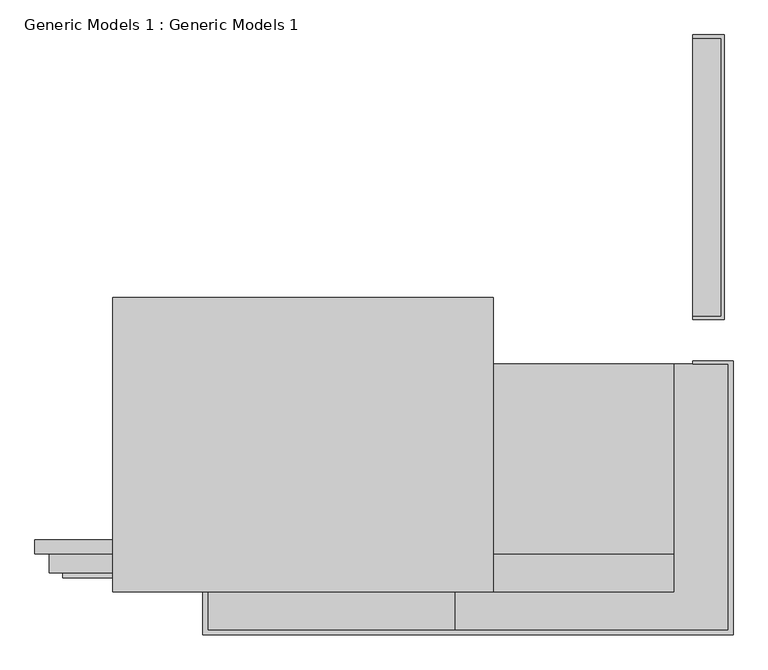
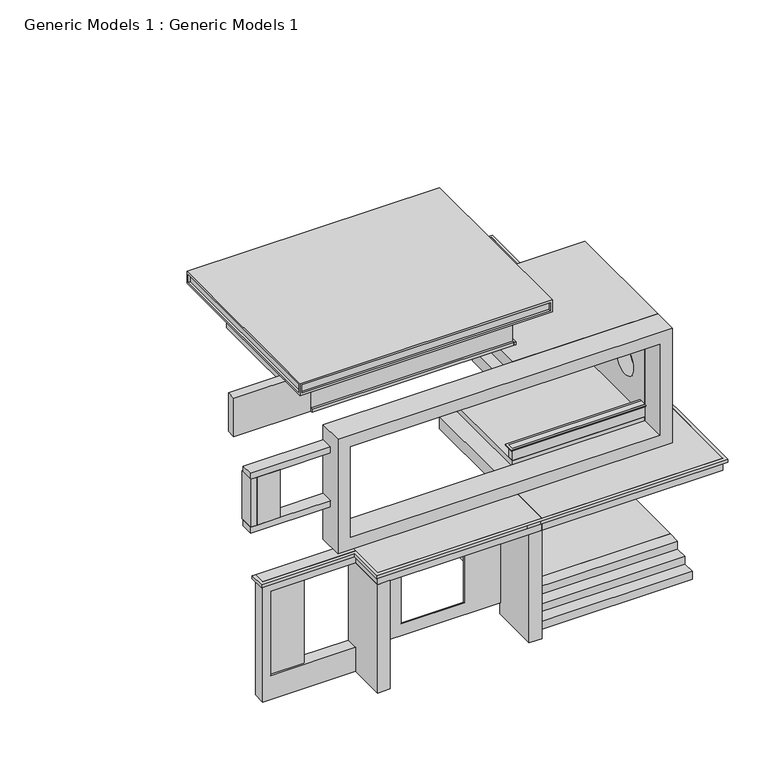
"""IFC4 building model written with IfcOpenShell, lengths in millimetres: proxy geometry, Generic Models 1 : Generic Models 1."""

from ifc_helpers import new_model, si_unit, point, frame, frame_2d, origin, place, context, project, spatial, polyline, circle_curve, trimmed, segment, composite_curve, outline, extrude, faceted_brep, source, transform, mapped, element, save


def generic_models_1_generic_models_1_6c446dcb(model_context):
    return source(origin(), model_context, "Body", "SolidModel", [
        extrude(outline(polyline([(-1556.9574339, 5927.1112267), (-1049.3218714, 5927.1112267), (-1049.3218714, 1362.7430362), (-1556.9574339, 1362.7430362), (-1556.9574339, 1413.5430362), (-1100.1218714, 1413.5430362), (-1100.1218714, 5876.3112267), (-1556.9574339, 5876.3112267), (-1556.9574339, 5927.1112267)])), frame((0.0, 0.0, 2969.3453176), z_axis=(0.0, 0.0, 1.0), x_axis=(1.0, 0.0, 0.0)), (0.0, 0.0, 1.0), 26.8742255),
        extrude(outline(polyline([(5876.0402075, 2996.2195432), (5876.0402075, 0.0), (1413.5430362, 0.0), (1413.5430362, 2996.2195432), (5876.0402075, 2996.2195432)]), holes=[polyline([(5571.2402075, 2691.4195432), (1718.3430362, 2691.4195432), (1718.3430362, 304.8), (5571.2402075, 304.8), (5571.2402075, 2691.4195432)])]), frame((-1557.3218714, 0.0, 0.0), z_axis=(1.0, 0.0, 0.0), x_axis=(0.0, 1.0, 0.0)), (0.0, 0.0, 1.0), 457.2),
        extrude(outline(polyline([(-2116.1218714, -2447.2569638), (-5418.1218714, -2447.2569638), (-5418.1218714, -2193.2569638), (-2116.1218714, -2193.2569638), (-2116.1218714, -2447.2569638)]), holes=[polyline([(-2166.9218714, -2244.0569638), (-5367.3218714, -2244.0569638), (-5367.3218714, -2396.4569638), (-2166.9218714, -2396.4569638), (-2166.9218714, -2244.0569638)])]), frame((0.0, 0.0, 4095.5509571), z_axis=(0.0, 0.0, 1.0), x_axis=(1.0, 0.0, 0.0)), (0.0, 0.0, 1.0), 30.3404478),
        extrude(outline(polyline([(-2166.9218714, -2244.0569638), (-2166.9218714, -2396.4569638), (-5367.3218714, -2396.4569638), (-5367.3218714, -2244.0569638), (-2166.9218714, -2244.0569638)])), frame((0.0, 0.0, 3810.0), z_axis=(0.0, 0.0, 1.0), x_axis=(1.0, 0.0, 0.0)), (0.0, 0.0, 1.0), 315.8914049),
        faceted_brep([(-10853.7218714, -3006.0569638, 8064.1157356), (-4757.7218714, -3006.0569638, 8064.1157356), (-4757.7218714, 1718.3430362, 8064.1157356), (-10853.7218714, 1718.3430362, 8064.1157356), (-10853.7218714, -3006.0569638, 7759.3157356), (-10853.7218714, 1718.3430362, 7759.3157356), (-4757.7218714, 1718.3430362, 7759.3157356), (-4757.7218714, -3006.0569638, 7759.3157356), (-4808.5218714, -3006.0569638, 8013.3157356), (-4808.5218714, -3006.0569638, 7810.1157356), (-10802.9218714, -3006.0569638, 7810.1157356), (-10802.9218714, -3006.0569638, 8013.3157356), (-4757.7218714, 1667.5430362, 8013.3157356), (-4757.7218714, 1667.5430362, 7810.1157356), (-4757.7218714, -2955.2569638, 7810.1157356), (-4757.7218714, -2955.2569638, 8013.3157356), (-10853.7218714, -2955.2569638, 8013.3157356), (-10853.7218714, -2955.2569638, 7810.1157356), (-10853.7218714, 1667.5430362, 7810.1157356), (-10853.7218714, 1667.5430362, 8013.3157356), (-4808.5218714, -2955.2569638, 8013.3157356), (-10802.9218714, -2955.2569638, 8013.3157356), (-10802.9218714, -2955.2569638, 7810.1157356), (-4808.5218714, -2955.2569638, 7810.1157356), (-4808.5218714, 1667.5430362, 8013.3157356), (-4808.5218714, -2955.2569638, 8013.3157356), (-4808.5218714, -2955.2569638, 7810.1157356), (-4808.5218714, 1667.5430362, 7810.1157356), (-10802.9218714, -2955.2569638, 8013.3157356), (-10802.9218714, 1667.5430362, 8013.3157356), (-10802.9218714, 1667.5430362, 7810.1157356), (-10802.9218714, -2955.2569638, 7810.1157356)], [[[0, 1, 2, 3]], [[4, 5, 6, 7]], [[1, 0, 4, 7], [8, 9, 10, 11]], [[2, 1, 7, 6], [12, 13, 14, 15]], [[3, 2, 6, 5]], [[0, 3, 5, 4], [16, 17, 18, 19]], [[20, 21, 22, 23]], [[20, 23, 9, 8]], [[23, 22, 10, 9]], [[22, 21, 11, 10]], [[21, 20, 8, 11]], [[24, 25, 26, 27]], [[24, 27, 13, 12]], [[27, 26, 14, 13]], [[26, 25, 15, 14]], [[25, 24, 12, 15]], [[28, 29, 30, 31]], [[28, 31, 17, 16]], [[31, 30, 18, 17]], [[30, 29, 19, 18]], [[29, 28, 16, 19]]]),
        extrude(outline(polyline([(-12098.3218714, -2396.4569638), (-12098.3218714, -2167.8569638), (-10244.1218714, -2167.8569638), (-10244.1218714, -2396.4569638), (-12098.3218714, -2396.4569638)])), frame((0.0, 0.0, 6776.5796237), z_axis=(0.0, 0.0, 1.0), x_axis=(1.0, 0.0, 0.0)), (0.0, 0.0, 1.0), 982.7361119),
        extrude(outline(polyline([(-5316.5218714, 651.5430362), (-5316.5218714, -2447.2569638), (-5367.3218714, -2447.2569638), (-5367.3218714, 651.5430362), (-5316.5218714, 651.5430362)])), frame((0.0, 0.0, 6776.5796237), z_axis=(0.0, 0.0, 1.0), x_axis=(1.0, 0.0, 0.0)), (0.0, 0.0, 1.0), 82.55),
        extrude(outline(polyline([(-5367.3218714, -2447.2569638), (-10244.1218714, -2447.2569638), (-10244.1218714, -2396.4569638), (-5367.3218714, -2396.4569638), (-5367.3218714, -2447.2569638)])), frame((0.0, 0.0, 6776.5796237), z_axis=(0.0, 0.0, 1.0), x_axis=(1.0, 0.0, 0.0)), (0.0, 0.0, 1.0), 81.4203763),
        extrude(outline(polyline([(-10244.1218714, -2396.4569638), (-10244.1218714, 1108.7430362), (-5367.3218714, 1108.7430362), (-5367.3218714, -2396.4569638), (-10244.1218714, -2396.4569638)]), holes=[polyline([(-10091.7218714, -2129.7569638), (-5634.0218714, -2129.7569638), (-5634.0218714, 870.1425368), (-10091.7218714, 870.1425368), (-10091.7218714, -2129.7569638)])]), frame((0.0, 0.0, 6776.5796237), z_axis=(0.0, 0.0, 1.0), x_axis=(1.0, 0.0, 0.0)), (0.0, 0.0, 1.0), 982.7361119),
        extrude(outline(polyline([(-11717.3218714, -2396.4569638), (-11158.5218714, -2396.4569638), (-11158.5218714, -2701.2569638), (-11717.3218714, -2701.2569638), (-11717.3218714, -2396.4569638)])), frame((0.0, 0.0, 4572.0), z_axis=(0.0, 0.0, 1.0), x_axis=(1.0, 0.0, 0.0)), (0.0, 0.0, 1.0), 1219.2),
        extrude(outline(polyline([(-11717.3218714, -2701.2569638), (-11869.7218714, -2701.2569638), (-11869.7218714, -2345.6569638), (-11717.3218714, -2345.6569638), (-11717.3218714, -2701.2569638)])), frame((0.0, 0.0, 4572.0), z_axis=(0.0, 0.0, 1.0), x_axis=(1.0, 0.0, 0.0)), (0.0, 0.0, 1.0), 1219.2),
        extrude(outline(polyline([(5943.6, -9939.3218714), (5943.6, -11869.7218714), (5791.2, -11869.7218714), (5791.2, -11158.5218714), (5791.2, -9939.3218714), (5943.6, -9939.3218714)])), frame((0.0, -2701.2569638, 0.0), z_axis=(0.0, 1.0, 0.0), x_axis=(0.0, 0.0, 1.0)), (0.0, 0.0, 1.0), 304.8),
        extrude(outline(polyline([(4419.6, -9939.3218714), (4572.0, -9939.3218714), (4572.0, -11158.5218714), (4572.0, -11869.7218714), (4419.6, -11869.7218714), (4419.6, -9939.3218714)])), frame((0.0, -2701.2569638, 0.0), z_axis=(0.0, 1.0, 0.0), x_axis=(0.0, 0.0, 1.0)), (0.0, 0.0, 1.0), 304.8),
        extrude(outline(polyline([(651.5430362, 3404.3806994), (-2396.4569638, 3404.3806994), (-2396.4569638, 6020.5806994), (651.5430362, 6020.5806994), (651.5430362, 3404.3806994)]), holes=[composite_curve([segment(trimmed(circle_curve(frame_2d((-1562.4008599, 4748.11296)), 355.6), [point((-1206.8008599, 4748.11296))], [point((-1918.0008599, 4748.11296))], True, "CARTESIAN"), True, "CONTINUOUS"), segment(trimmed(circle_curve(frame_2d((-1562.4008599, 4748.11296)), 355.6), [point((-1918.0008599, 4748.11296))], [point((-1206.8008599, 4748.11296))], True, "CARTESIAN"), True, "CONTINUOUS")], self_intersect=False)]), frame((-2166.9218714, 0.0, 0.0), z_axis=(1.0, 0.0, 0.0), x_axis=(0.0, 1.0, 0.0)), (0.0, 0.0, 1.0), 304.8),
        extrude(outline(polyline([(-1862.1218714, -2396.4569638), (-5367.3218714, -2396.4569638), (-5367.3218714, 651.5430362), (-1862.1218714, 651.5430362), (-1862.1218714, -2396.4569638)])), frame((0.0, 0.0, 6020.5806994), z_axis=(0.0, 0.0, 1.0), x_axis=(1.0, 0.0, 0.0)), (0.0, 0.0, 1.0), 304.8),
        extrude(outline(polyline([(-2166.9218714, 651.5430362), (-2166.9218714, -2396.4569638), (-5367.3218714, -2396.4569638), (-5367.3218714, 651.5430362), (-2166.9218714, 651.5430362)])), frame((0.0, 0.0, 3657.6), z_axis=(0.0, 0.0, 1.0), x_axis=(1.0, 0.0, 0.0)), (0.0, 0.0, 1.0), 152.4),
        extrude(outline(polyline([(3404.3806994, -1862.1218714), (6325.3806994, -1862.1218714), (6325.3806994, -9939.3218714), (3404.3806994, -9939.3218714), (3404.3806994, -1862.1218714)]), holes=[polyline([(3709.1806994, -2166.9218714), (3709.1806994, -9634.5218714), (6020.5806994, -9634.5218714), (6020.5806994, -2166.9218714), (3709.1806994, -2166.9218714)])]), frame((0.0, -3006.0569638, 0.0), z_axis=(0.0, 1.0, 0.0), x_axis=(0.0, 0.0, 1.0)), (0.0, 0.0, 1.0), 609.6),
        extrude(outline(polyline([(-6548.4218714, -2421.8569638), (-8072.4218714, -2421.8569638), (-8072.4218714, -2396.4569638), (-6548.4218714, -2396.4569638), (-6548.4218714, -2421.8569638)])), frame((0.0, 0.0, 2743.9806994), z_axis=(0.0, 0.0, 1.0), x_axis=(1.0, 0.0, 0.0)), (0.0, 0.0, 1.0), 25.4),
        extrude(outline(polyline([(305.5806994, -9024.9218714), (305.5806994, -5672.1218714), (2769.3806994, -5672.1218714), (2769.3806994, -6548.4218714), (610.3806994, -6548.4218714), (610.3806994, -8072.4218714), (2769.3806994, -8072.4218714), (2769.3806994, -9024.9218714), (305.5806994, -9024.9218714)])), frame((0.0, -2421.8569638, 0.0), z_axis=(0.0, 1.0, 0.0), x_axis=(0.0, 0.0, 1.0)), (0.0, 0.0, 1.0), 25.4),
        extrude(outline(polyline([(-911.5185038, -3691.8569638), (-5443.5218714, -3691.8569638), (-5765.5707624, -3691.8569638), (-9405.9218714, -3691.8569638), (-9405.9218714, -2777.4569638), (-11653.8218714, -2777.4569638), (-11653.8218714, -2396.4569638), (-11577.6218714, -2396.4569638), (-11577.6218714, -2701.2569638), (-9329.7218714, -2701.2569638), (-9329.7218714, -3615.6569638), (-5367.3218714, -3615.6569638), (-987.7185038, -3615.6569638), (-987.7185038, 651.5430362), (-1557.3218714, 651.5430362), (-1557.3218714, 702.3430362), (-911.5185038, 702.3430362), (-911.5185038, -3691.8569638)])), frame((0.0, 0.0, 2996.2195432), z_axis=(0.0, 0.0, 1.0), x_axis=(1.0, 0.0, 0.0)), (0.0, 0.0, 1.0), 77.9611562),
        faceted_brep([(-11577.6218714, -2701.2569638, 3074.1806994), (-11577.6218714, -2701.2569638, 0.7806994), (-9329.7218714, -2701.2569638, 0.7806994), (-9329.7218714, -2701.2569638, 610.3806994), (-11388.5601903, -2701.2569638, 610.3806994), (-11388.5601903, -2701.2569638, 2769.3806994), (-9329.7218714, -2701.2569638, 2769.3806994), (-9329.7218714, -2701.2569638, 3074.1806994), (-11577.6218714, -2396.4569638, 3074.1806994), (-9329.7218714, -2396.4569638, 3074.1806994), (-9329.7218714, -2396.4569638, 2769.3806994), (-10548.9218714, -2396.4569638, 2769.3806994), (-10548.9218714, -2396.4569638, 610.3806994), (-9329.7218714, -2396.4569638, 610.3806994), (-9329.7218714, -2396.4569638, 0.7806994), (-11577.6218714, -2396.4569638, 0.7806994), (-11388.5601903, -2650.4569638, 2769.3806994), (-10548.9218714, -2650.4569638, 2769.3806994), (-10548.9218714, -2650.4569638, 610.3806994), (-11388.5601903, -2650.4569638, 610.3806994)], [[[0, 1, 2, 3, 4, 5, 6, 7]], [[8, 9, 10, 11, 12, 13, 14, 15]], [[1, 0, 8, 15]], [[2, 1, 15, 14]], [[3, 2, 14, 13]], [[0, 7, 9, 8]], [[11, 10, 6, 5, 16, 17]], [[13, 12, 18, 19, 4, 3]], [[12, 11, 17, 18]], [[7, 6, 10, 9]], [[16, 19, 18, 17]], [[19, 16, 5, 4]]]),
        extrude(outline(polyline([(-9024.9218714, -3615.6569638), (-9329.7218714, -3615.6569638), (-9329.7218714, -2396.4569638), (-9024.9218714, -2396.4569638), (-9024.9218714, -3615.6569638)])), frame((0.0, 0.0, 0.7806994), z_axis=(0.0, 0.0, 1.0), x_axis=(1.0, 0.0, 0.0)), (0.0, 0.0, 1.0), 2768.6),
        extrude(outline(polyline([(-9329.7218714, -3615.6569638), (-9329.7218714, -2396.4569638), (-5367.3218714, -2396.4569638), (-5367.3218714, -3615.6569638), (-9329.7218714, -3615.6569638)])), frame((0.0, 0.0, 2769.3806994), z_axis=(0.0, 0.0, 1.0), x_axis=(1.0, 0.0, 0.0)), (0.0, 0.0, 1.0), 304.8),
        extrude(outline(polyline([(-987.7185038, 651.5430362), (-987.7185038, -3615.6569638), (-5367.3218714, -3615.6569638), (-5367.3218714, 651.5430362), (-987.7185038, 651.5430362)])), frame((0.0, 0.0, 2769.3806994), z_axis=(0.0, 0.0, 1.0), x_axis=(1.0, 0.0, 0.0)), (0.0, 0.0, 1.0), 304.8),
        extrude(outline(polyline([(-5367.3218714, -3615.6569638), (-5672.1218714, -3615.6569638), (-5672.1218714, -2396.4569638), (-5367.3218714, -2396.4569638), (-5367.3218714, -3615.6569638)])), frame((0.0, 0.0, 0.7806994), z_axis=(0.0, 0.0, 1.0), x_axis=(1.0, 0.0, 0.0)), (0.0, 0.0, 1.0), 2768.6),
        extrude(outline(polyline([(-2396.4569638, 605.6987522), (-2396.4569638, 0.7806994), (-3310.8569638, 0.7806994), (-3310.8569638, 199.2987522), (-3006.0569638, 199.2987522), (-3006.0569638, 402.4987522), (-2701.2569638, 402.4987522), (-2701.2569638, 605.6987522), (-2396.4569638, 605.6987522)])), frame((-5367.3218714, 0.0, 0.0), z_axis=(1.0, 0.0, 0.0), x_axis=(0.0, 1.0, 0.0)), (0.0, 0.0, 1.0), 3810.0),
        extrude(outline(polyline([(-1557.3218714, 651.5430362), (-1557.3218714, -2396.4569638), (-5367.3218714, -2396.4569638), (-5367.3218714, 651.5430362), (-1557.3218714, 651.5430362)])), frame((0.0, 0.0, -3.9012478), z_axis=(0.0, 0.0, 1.0), x_axis=(1.0, 0.0, 0.0)), (0.0, 0.0, 1.0), 609.6),
    ])


if __name__ == "__main__":
    model = new_model("IFC4")
    model_context = context("Model", 3, world=origin())
    ifc_project = project(units=[si_unit("LENGTHUNIT", "METRE", prefix="MILLI")], contexts=[model_context])
    site = spatial("IfcSite", under=ifc_project)
    building = spatial("IfcBuilding", under=site)
    placement = place(None, origin())
    generic_models_1_generic_models_1_shape = generic_models_1_generic_models_1_6c446dcb(model_context)
    element("IfcBuildingElementProxy", 1, Name="Generic Models 1 : Generic Models 1", ObjectType="Generic Models 1 : Generic Models 1", at=placement, inside=building, context=model_context, shape_type="MappedRepresentation", body=[
        mapped(generic_models_1_generic_models_1_shape, transform((0.0, 0.0, 0.0), x_axis=(1.0, 0.0, 0.0), y_axis=(0.0, 1.0, 0.0), z_axis=(0.0, 0.0, 1.0))),
    ])
    save(model, "model.ifc")

# Revit data of these elements
# Element 1 (IfcBuildingElementProxy, "Generic Models 1 : Generic Models 1")
#   Materials on its faces: "Gypsum Wall Board", "Earth", "Wood - Stained", "wood colour", "wall wood"
# Materials
#   "Gypsum Wall Board": class "Generic", colour RGB 127 127 127, transparency 0, Description = "Gypsum Wall Board", Cost = 0
#   "Earth": class "Generic", colour RGB 97 75 62, transparency 0, Description = "Soil", Cost = 0
#   "Wood - Stained": class "Wood", colour RGB 224 178 126, transparency 0, Cost = 0
#   "wood colour": class "Generic", colour RGB 120 120 120, transparency 0, Cost = 0
#   "wall wood": class "Generic", colour RGB 120 120 120, transparency 0, Cost = 0
